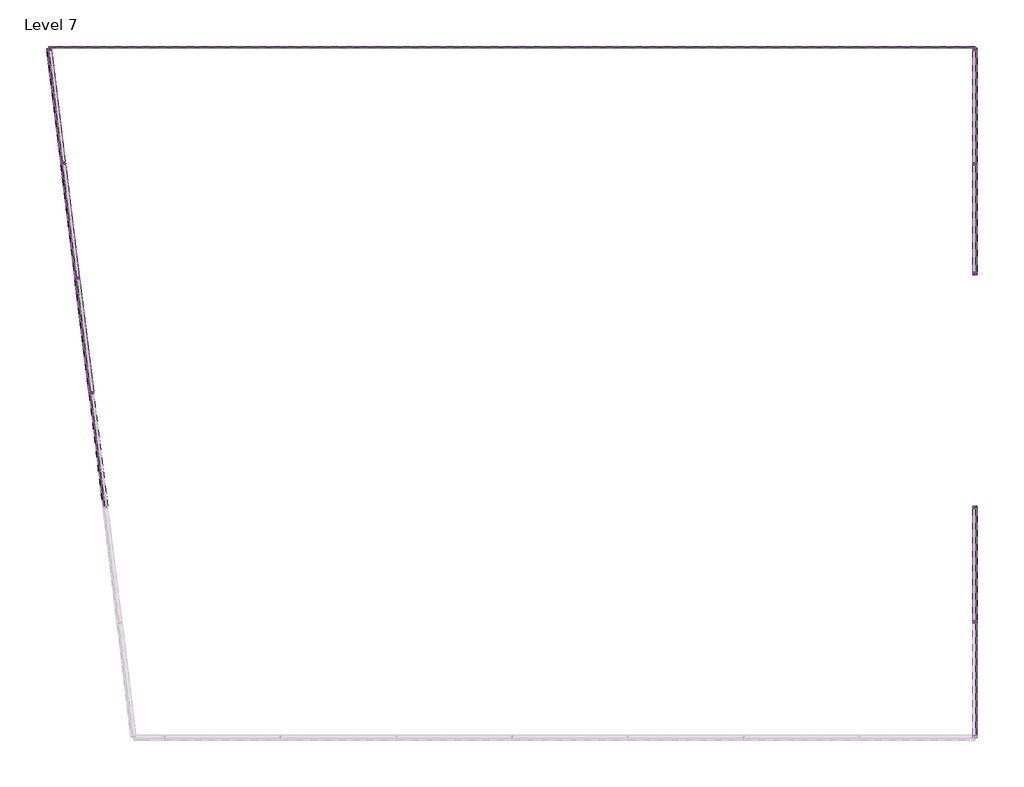
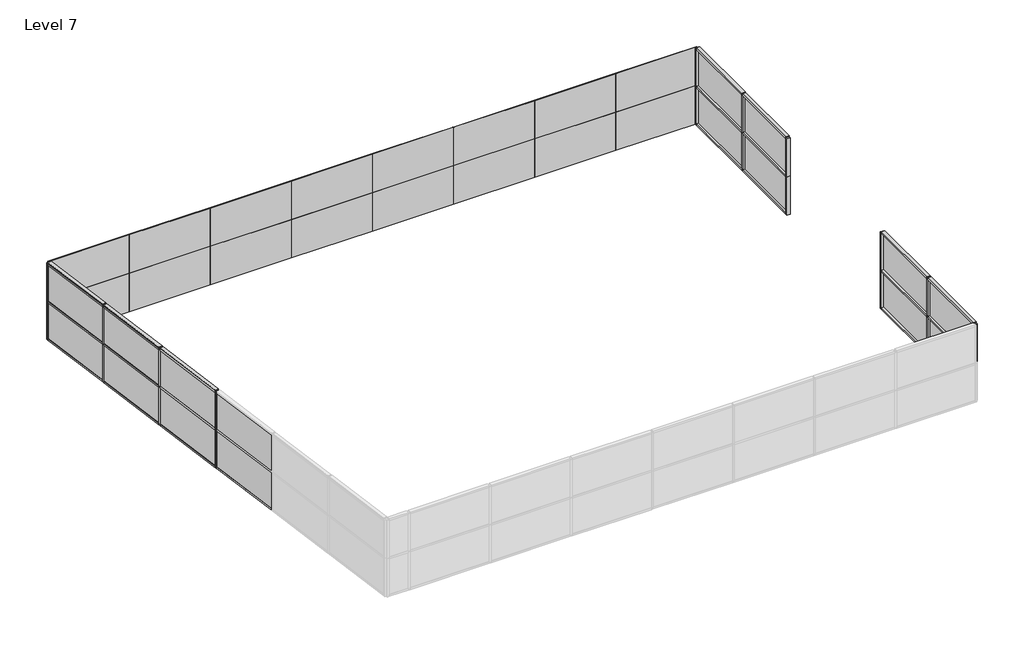
# One storey, part 2 of 2: 54 members, 40 plates.
"""IFC4 building model written with IfcOpenShell, lengths in millimetres."""

from ifc_helpers import new_model, si_unit, origin, place, context, project, spatial, transform, mapped, element, save
from components import member_71c27fd2, member_daa7a266, member_82905deb, member_19d0a4ec, member_8cef0660, member_db480205, member_4491d118, member_1b94d493, member_46bdb8c2, system_panel_glazed_1e57f9bb, system_panel_glazed_37f15d2e, system_panel_glazed_3620f98e, system_panel_glazed_e46d4b42, system_panel_glazed_2a6c68b7, system_panel_glazed_7fb1fc2b, system_panel_glazed_d483336f

model = new_model("IFC4")

# Units and contexts
model_context = context("Model", 3, world=origin())
ifc_project = project(units=[si_unit("LENGTHUNIT", "METRE", prefix="MILLI")], contexts=[model_context])

# Site, building, storey
site = spatial("IfcSite", under=ifc_project)
building = spatial("IfcBuilding", under=site)
storey = spatial("IfcBuildingStorey", under=building, Name="Level 7", Elevation=18288.0)

# Members
placement = place(None, origin())
member_shape = member_71c27fd2(model_context)
element("IfcMember", 1, ObjectType="Rectangular Mullion : 2.5\" x 5\" rectangular", at=placement, inside=storey, context=model_context, shape_type="MappedRepresentation", body=[
    mapped(member_shape, transform((-10473.7456604, 11109.5209701, 18288.0), x_axis=(0.0, 0.0, -1.0), y_axis=(-0.9925461516413222, -0.12186934340514599, 0.0), z_axis=(-0.12186934340514599, 0.9925461516413222, 0.0))),
])
element("IfcMember", 2, ObjectType="Rectangular Mullion : 2.5\" x 5\" rectangular", at=placement, inside=storey, context=model_context, shape_type="MappedRepresentation", body=[
    mapped(member_shape, transform((13902.5156363, -3899.3863708, 18288.0), x_axis=(0.0, 0.0, -1.0), y_axis=(1.0, 0.0, 0.0), z_axis=(0.0, -1.0, 0.0))),
])
element("IfcMember", 3, ObjectType="Rectangular Mullion : 2.5\" x 5\" rectangular", at=placement, inside=storey, context=model_context, shape_type="MappedRepresentation", body=[
    mapped(member_shape, transform((13902.5156363, 8156.2976505, 18288.0), x_axis=(0.0, 0.0, -1.0), y_axis=(1.0, 0.0, 0.0), z_axis=(0.0, -1.0, 0.0))),
])
member_2_shape = member_daa7a266(model_context)
element("IfcMember", 4, ObjectType="Rectangular Mullion : 2.5\" x 5\" rectangular", at=placement, inside=storey, context=model_context, shape_type="MappedRepresentation", body=[
    mapped(member_2_shape, transform((-10113.8959567, 8178.7803212, 21336.0), x_axis=(0.0, 0.0, 1.0), y_axis=(-0.9925461516413222, -0.12186934340514625, 0.0), z_axis=(0.12186934340514625, -0.9925461516413222, 0.0))),
])
member_3_shape = member_82905deb(model_context)
element("IfcMember", 5, ObjectType="Rectangular Mullion : 2.5\" x 5\" rectangular", at=placement, inside=storey, context=model_context, shape_type="MappedRepresentation", body=[
    mapped(member_3_shape, transform((-9367.1110876, 2096.7056405, 21336.0), x_axis=(-0.1218693434051459, 0.9925461516413222, 0.0), y_axis=(-0.9925461516413222, -0.1218693434051459, 0.0), z_axis=(0.0, 0.0, 1.0))),
])
element("IfcMember", 6, ObjectType="Rectangular Mullion : 2.5\" x 5\" rectangular", at=placement, inside=storey, context=model_context, shape_type="MappedRepresentation", body=[
    mapped(member_3_shape, transform((-9738.5688463, 5121.9863107, 21336.0), x_axis=(-0.1218693434051459, 0.9925461516413222, 0.0), y_axis=(-0.9925461516413222, -0.1218693434051459, 0.0), z_axis=(0.0, 0.0, 1.0))),
])
element("IfcMember", 7, ObjectType="Rectangular Mullion : 2.5\" x 5\" rectangular", at=placement, inside=storey, context=model_context, shape_type="MappedRepresentation", body=[
    mapped(member_3_shape, transform((-10110.026605, 8147.2669809, 21336.0), x_axis=(-0.1218693434051459, 0.9925461516413222, 0.0), y_axis=(-0.9925461516413222, -0.1218693434051459, 0.0), z_axis=(0.0, 0.0, 1.0))),
])
member_4_shape = member_19d0a4ec(model_context)
element("IfcMember", 8, ObjectType="Rectangular Mullion : 2.5\" x 5\" rectangular", at=placement, inside=storey, context=model_context, shape_type="MappedRepresentation", body=[
    mapped(member_4_shape, transform((-10113.8959567, 8178.7803212, 19812.0), x_axis=(0.0, 0.0, 1.0), y_axis=(-0.9925461516413223, -0.12186934340514552, 0.0), z_axis=(0.1218693434051455, -0.9925461516413222, 0.0))),
])
element("IfcMember", 9, ObjectType="Rectangular Mullion : 2.5\" x 5\" rectangular", at=placement, inside=storey, context=model_context, shape_type="MappedRepresentation", body=[
    mapped(member_4_shape, transform((-10113.8959567, 8178.7803212, 19812.0), x_axis=(0.0, 0.0, 1.0), y_axis=(-0.9925461516413222, -0.12186934340514599, 0.0), z_axis=(0.12186934340514599, -0.9925461516413222, 0.0))),
])
element("IfcMember", 10, ObjectType="Rectangular Mullion : 2.5\" x 5\" rectangular", at=placement, inside=storey, context=model_context, shape_type="MappedRepresentation", body=[
    mapped(member_4_shape, transform((-10113.8959567, 8178.7803212, 21336.0), x_axis=(0.0, 0.0, 1.0), y_axis=(-0.9925461516413222, -0.12186934340514599, 0.0), z_axis=(0.12186934340514599, -0.9925461516413222, 0.0))),
])
element("IfcMember", 11, ObjectType="Rectangular Mullion : 2.5\" x 5\" rectangular", at=placement, inside=storey, context=model_context, shape_type="MappedRepresentation", body=[
    mapped(member_4_shape, transform((13902.5156363, -946.6363705, 19812.0), x_axis=(0.0, 0.0, 1.0), y_axis=(1.0, 0.0, 0.0), z_axis=(0.0, 1.0, 0.0))),
])
element("IfcMember", 12, ObjectType="Rectangular Mullion : 2.5\" x 5\" rectangular", at=placement, inside=storey, context=model_context, shape_type="MappedRepresentation", body=[
    mapped(member_4_shape, transform((13902.5156363, -3962.8863708, 19812.0), x_axis=(0.0, 0.0, 1.0), y_axis=(1.0, 0.0, 0.0), z_axis=(0.0, 1.0, 0.0))),
])
element("IfcMember", 13, ObjectType="Rectangular Mullion : 2.5\" x 5\" rectangular", at=placement, inside=storey, context=model_context, shape_type="MappedRepresentation", body=[
    mapped(member_4_shape, transform((13902.5156363, -946.6363705, 21336.0), x_axis=(0.0, 0.0, 1.0), y_axis=(1.0, 0.0, 0.0), z_axis=(0.0, 1.0, 0.0))),
])
element("IfcMember", 14, ObjectType="Rectangular Mullion : 2.5\" x 5\" rectangular", at=placement, inside=storey, context=model_context, shape_type="MappedRepresentation", body=[
    mapped(member_4_shape, transform((13902.5156363, -3962.8863708, 21336.0), x_axis=(0.0, 0.0, 1.0), y_axis=(1.0, 0.0, 0.0), z_axis=(0.0, 1.0, 0.0))),
])
element("IfcMember", 15, ObjectType="Rectangular Mullion : 2.5\" x 5\" rectangular", at=placement, inside=storey, context=model_context, shape_type="MappedRepresentation", body=[
    mapped(member_4_shape, transform((13902.5156363, 11109.0476508, 19812.0), x_axis=(0.0, 0.0, 1.0), y_axis=(1.0, 0.0, 0.0), z_axis=(0.0, 1.0, 0.0))),
])
element("IfcMember", 16, ObjectType="Rectangular Mullion : 2.5\" x 5\" rectangular", at=placement, inside=storey, context=model_context, shape_type="MappedRepresentation", body=[
    mapped(member_4_shape, transform((13902.5156363, 11109.0476508, 21336.0), x_axis=(0.0, 0.0, 1.0), y_axis=(1.0, 0.0, 0.0), z_axis=(0.0, 1.0, 0.0))),
])
member_5_shape = member_8cef0660(model_context)
element("IfcMember", 17, ObjectType="Rectangular Mullion : 2.5\" x 5\" rectangular", at=placement, inside=storey, context=model_context, shape_type="MappedRepresentation", body=[
    mapped(member_5_shape, transform((-9370.9804393, 2128.2189808, 19812.0), x_axis=(0.0, 0.0, 1.0), y_axis=(-0.9925461516413222, -0.12186934340514592, 0.0), z_axis=(0.12186934340514592, -0.9925461516413222, 0.0))),
])
element("IfcMember", 18, ObjectType="Rectangular Mullion : 2.5\" x 5\" rectangular", at=placement, inside=storey, context=model_context, shape_type="MappedRepresentation", body=[
    mapped(member_5_shape, transform((-9742.438198, 5153.499651, 19812.0), x_axis=(0.0, 0.0, 1.0), y_axis=(-0.9925461516413222, -0.12186934340514602, 0.0), z_axis=(0.12186934340514602, -0.9925461516413222, 0.0))),
])
element("IfcMember", 19, ObjectType="Rectangular Mullion : 2.5\" x 5\" rectangular", at=placement, inside=storey, context=model_context, shape_type="MappedRepresentation", body=[
    mapped(member_5_shape, transform((-9370.9804393, 2128.2189808, 19812.0), x_axis=(0.0, 0.0, 1.0), y_axis=(-0.9925461516413222, -0.12186934340514592, 0.0), z_axis=(0.12186934340514592, -0.9925461516413222, 0.0))),
])
element("IfcMember", 20, ObjectType="Rectangular Mullion : 2.5\" x 5\" rectangular", at=placement, inside=storey, context=model_context, shape_type="MappedRepresentation", body=[
    mapped(member_5_shape, transform((-9742.438198, 5153.499651, 19812.0), x_axis=(0.0, 0.0, 1.0), y_axis=(-0.9925461516413222, -0.1218693434051457, 0.0), z_axis=(0.1218693434051457, -0.9925461516413222, 0.0))),
])
element("IfcMember", 21, ObjectType="Rectangular Mullion : 2.5\" x 5\" rectangular", at=placement, inside=storey, context=model_context, shape_type="MappedRepresentation", body=[
    mapped(member_5_shape, transform((-9370.9804393, 2128.2189808, 21336.0), x_axis=(0.0, 0.0, 1.0), y_axis=(-0.9925461516413222, -0.12186934340514595, 0.0), z_axis=(0.12186934340514595, -0.9925461516413222, 0.0))),
])
element("IfcMember", 22, ObjectType="Rectangular Mullion : 2.5\" x 5\" rectangular", at=placement, inside=storey, context=model_context, shape_type="MappedRepresentation", body=[
    mapped(member_5_shape, transform((-9742.438198, 5153.499651, 21336.0), x_axis=(0.0, 0.0, 1.0), y_axis=(-0.9925461516413222, -0.12186934340514606, 0.0), z_axis=(0.12186934340514606, -0.9925461516413222, 0.0))),
])
member_6_shape = member_db480205(model_context)
element("IfcMember", 23, ObjectType="Rectangular Mullion : 2.5\" x 5\" rectangular", at=placement, inside=storey, context=model_context, shape_type="MappedRepresentation", body=[
    mapped(member_6_shape, transform((-9363.241736, 2065.1923001, 18288.0), x_axis=(0.0, 0.0, -1.0), y_axis=(-0.9925461516413223, -0.12186934340514559, 0.0), z_axis=(-0.12186934340514559, 0.9925461516413223, 0.0))),
])
element("IfcMember", 24, ObjectType="Rectangular Mullion : 2.5\" x 5\" rectangular", at=placement, inside=storey, context=model_context, shape_type="MappedRepresentation", body=[
    mapped(member_6_shape, transform((-9734.6994947, 5090.4729703, 18288.0), x_axis=(0.0, 0.0, -1.0), y_axis=(-0.9925461516413222, -0.12186934340514592, 0.0), z_axis=(-0.12186934340514592, 0.9925461516413222, 0.0))),
])
element("IfcMember", 25, ObjectType="Rectangular Mullion : 2.5\" x 5\" rectangular", at=placement, inside=storey, context=model_context, shape_type="MappedRepresentation", body=[
    mapped(member_6_shape, transform((-10106.1572534, 8115.7536405, 18288.0), x_axis=(0.0, 0.0, -1.0), y_axis=(-0.9925461516413222, -0.12186934340514606, 0.0), z_axis=(-0.12186934340514606, 0.9925461516413222, 0.0))),
])
element("IfcMember", 26, ObjectType="Rectangular Mullion : 2.5\" x 5\" rectangular", at=placement, inside=storey, context=model_context, shape_type="MappedRepresentation", body=[
    mapped(member_6_shape, transform((-9370.9804393, 2128.2189808, 21336.0), x_axis=(0.0, 0.0, 1.0), y_axis=(-0.9925461516413222, -0.12186934340514592, 0.0), z_axis=(0.12186934340514592, -0.9925461516413222, 0.0))),
])
element("IfcMember", 27, ObjectType="Rectangular Mullion : 2.5\" x 5\" rectangular", at=placement, inside=storey, context=model_context, shape_type="MappedRepresentation", body=[
    mapped(member_6_shape, transform((-9742.438198, 5153.499651, 21336.0), x_axis=(0.0, 0.0, 1.0), y_axis=(-0.9925461516413222, -0.1218693434051457, 0.0), z_axis=(0.1218693434051457, -0.9925461516413222, 0.0))),
])
element("IfcMember", 28, ObjectType="Rectangular Mullion : 2.5\" x 5\" rectangular", at=placement, inside=storey, context=model_context, shape_type="MappedRepresentation", body=[
    mapped(member_3_shape, transform((-9367.1110876, 2096.7056405, 19812.0), x_axis=(-0.1218693434051459, 0.9925461516413222, 0.0), y_axis=(-0.9925461516413222, -0.1218693434051459, 0.0), z_axis=(0.0, 0.0, 1.0))),
])
element("IfcMember", 29, ObjectType="Rectangular Mullion : 2.5\" x 5\" rectangular", at=placement, inside=storey, context=model_context, shape_type="MappedRepresentation", body=[
    mapped(member_3_shape, transform((-9738.5688463, 5121.9863107, 19812.0), x_axis=(-0.1218693434051459, 0.9925461516413222, 0.0), y_axis=(-0.9925461516413222, -0.1218693434051459, 0.0), z_axis=(0.0, 0.0, 1.0))),
])
element("IfcMember", 30, ObjectType="Rectangular Mullion : 2.5\" x 5\" rectangular", at=placement, inside=storey, context=model_context, shape_type="MappedRepresentation", body=[
    mapped(member_3_shape, transform((-10110.026605, 8147.2669809, 19812.0), x_axis=(-0.1218693434051459, 0.9925461516413222, 0.0), y_axis=(-0.9925461516413222, -0.1218693434051459, 0.0), z_axis=(0.0, 0.0, 1.0))),
])
element("IfcMember", 31, ObjectType="Rectangular Mullion : 2.5\" x 5\" rectangular", at=placement, inside=storey, context=model_context, shape_type="MappedRepresentation", body=[
    mapped(member_3_shape, transform((13902.5156363, -3931.1363708, 19812.0), x_axis=(0.0, -1.0, 0.0), y_axis=(1.0, 0.0, 0.0), z_axis=(0.0, 0.0, 1.0))),
])
element("IfcMember", 32, ObjectType="Rectangular Mullion : 2.5\" x 5\" rectangular", at=placement, inside=storey, context=model_context, shape_type="MappedRepresentation", body=[
    mapped(member_3_shape, transform((13902.5156363, 8124.5476505, 19812.0), x_axis=(0.0, -1.0, 0.0), y_axis=(1.0, 0.0, 0.0), z_axis=(0.0, 0.0, 1.0))),
])
element("IfcMember", 33, ObjectType="Rectangular Mullion : 2.5\" x 5\" rectangular", at=placement, inside=storey, context=model_context, shape_type="MappedRepresentation", body=[
    mapped(member_3_shape, transform((-9367.1110876, 2096.7056405, 19812.0), x_axis=(-0.1218693434051459, 0.9925461516413222, 0.0), y_axis=(-0.9925461516413222, -0.1218693434051459, 0.0), z_axis=(0.0, 0.0, 1.0))),
])
element("IfcMember", 34, ObjectType="Rectangular Mullion : 2.5\" x 5\" rectangular", at=placement, inside=storey, context=model_context, shape_type="MappedRepresentation", body=[
    mapped(member_3_shape, transform((-9738.5688463, 5121.9863107, 19812.0), x_axis=(-0.1218693434051459, 0.9925461516413222, 0.0), y_axis=(-0.9925461516413222, -0.1218693434051459, 0.0), z_axis=(0.0, 0.0, 1.0))),
])
element("IfcMember", 35, ObjectType="Rectangular Mullion : 2.5\" x 5\" rectangular", at=placement, inside=storey, context=model_context, shape_type="MappedRepresentation", body=[
    mapped(member_3_shape, transform((-10110.026605, 8147.2669809, 19812.0), x_axis=(-0.1218693434051459, 0.9925461516413222, 0.0), y_axis=(-0.9925461516413222, -0.1218693434051459, 0.0), z_axis=(0.0, 0.0, 1.0))),
])
element("IfcMember", 36, ObjectType="Rectangular Mullion : 2.5\" x 5\" rectangular", at=placement, inside=storey, context=model_context, shape_type="MappedRepresentation", body=[
    mapped(member_3_shape, transform((-9367.1110876, 2096.7056405, 21336.0), x_axis=(-0.1218693434051459, 0.9925461516413222, 0.0), y_axis=(-0.9925461516413222, -0.1218693434051459, 0.0), z_axis=(0.0, 0.0, 1.0))),
])
element("IfcMember", 37, ObjectType="Rectangular Mullion : 2.5\" x 5\" rectangular", at=placement, inside=storey, context=model_context, shape_type="MappedRepresentation", body=[
    mapped(member_3_shape, transform((-9738.5688463, 5121.9863107, 21336.0), x_axis=(-0.1218693434051459, 0.9925461516413222, 0.0), y_axis=(-0.9925461516413222, -0.1218693434051459, 0.0), z_axis=(0.0, 0.0, 1.0))),
])
element("IfcMember", 38, ObjectType="Rectangular Mullion : 2.5\" x 5\" rectangular", at=placement, inside=storey, context=model_context, shape_type="MappedRepresentation", body=[
    mapped(member_3_shape, transform((-10110.026605, 8147.2669809, 21336.0), x_axis=(-0.1218693434051459, 0.9925461516413222, 0.0), y_axis=(-0.9925461516413222, -0.1218693434051459, 0.0), z_axis=(0.0, 0.0, 1.0))),
])
element("IfcMember", 39, ObjectType="Rectangular Mullion : 2.5\" x 5\" rectangular", at=placement, inside=storey, context=model_context, shape_type="MappedRepresentation", body=[
    mapped(member_3_shape, transform((13902.5156363, -3931.1363708, 21336.0), x_axis=(0.0, -1.0, 0.0), y_axis=(1.0, 0.0, 0.0), z_axis=(0.0, 0.0, 1.0))),
])
element("IfcMember", 40, ObjectType="Rectangular Mullion : 2.5\" x 5\" rectangular", at=placement, inside=storey, context=model_context, shape_type="MappedRepresentation", body=[
    mapped(member_3_shape, transform((13902.5156363, 8124.5476505, 21336.0), x_axis=(0.0, -1.0, 0.0), y_axis=(1.0, 0.0, 0.0), z_axis=(0.0, 0.0, 1.0))),
])
member_7_shape = member_4491d118(model_context)
element("IfcMember", 41, ObjectType="Rectangular Mullion : 2.5\" x 5\" rectangular", at=placement, inside=storey, context=model_context, shape_type="MappedRepresentation", body=[
    mapped(member_7_shape, transform((-10481.4843637, 11172.5476508, 21336.0), x_axis=(-0.1218693434051459, 0.9925461516413222, 0.0), y_axis=(-0.9925461516413222, -0.1218693434051459, 0.0), z_axis=(0.0, 0.0, 1.0))),
])
element("IfcMember", 42, ObjectType="Rectangular Mullion : 2.5\" x 5\" rectangular", at=placement, inside=storey, context=model_context, shape_type="MappedRepresentation", body=[
    mapped(member_7_shape, transform((13902.5156363, -883.1363705, 18288.0), x_axis=(0.0, 1.0, 0.0), y_axis=(1.0, 0.0, 0.0), z_axis=(0.0, 0.0, -1.0))),
])
element("IfcMember", 43, ObjectType="Rectangular Mullion : 2.5\" x 5\" rectangular", at=placement, inside=storey, context=model_context, shape_type="MappedRepresentation", body=[
    mapped(member_7_shape, transform((13902.5156363, 11172.5476508, 18288.0), x_axis=(0.0, 1.0, 0.0), y_axis=(1.0, 0.0, 0.0), z_axis=(0.0, 0.0, -1.0))),
])
element("IfcMember", 44, ObjectType="Rectangular Mullion : 2.5\" x 5\" rectangular", at=placement, inside=storey, context=model_context, shape_type="MappedRepresentation", body=[
    mapped(member_7_shape, transform((13902.5156363, -883.1363705, 19812.0), x_axis=(0.0, 1.0, 0.0), y_axis=(1.0, 0.0, 0.0), z_axis=(0.0, 0.0, -1.0))),
])
element("IfcMember", 45, ObjectType="Rectangular Mullion : 2.5\" x 5\" rectangular", at=placement, inside=storey, context=model_context, shape_type="MappedRepresentation", body=[
    mapped(member_7_shape, transform((13902.5156363, 11172.5476508, 19812.0), x_axis=(0.0, 1.0, 0.0), y_axis=(1.0, 0.0, 0.0), z_axis=(0.0, 0.0, -1.0))),
])
element("IfcMember", 46, ObjectType="Rectangular Mullion : 2.5\" x 5\" rectangular", at=placement, inside=storey, context=model_context, shape_type="MappedRepresentation", body=[
    mapped(member_7_shape, transform((-10481.4843637, 11172.5476508, 19812.0), x_axis=(-0.1218693434051459, 0.9925461516413222, 0.0), y_axis=(-0.9925461516413222, -0.1218693434051459, 0.0), z_axis=(0.0, 0.0, 1.0))),
])
element("IfcMember", 47, ObjectType="Rectangular Mullion : 2.5\" x 5\" rectangular", at=placement, inside=storey, context=model_context, shape_type="MappedRepresentation", body=[
    mapped(member_7_shape, transform((13902.5156363, 5212.8636295, 19812.0), x_axis=(0.0, -1.0, 0.0), y_axis=(1.0, 0.0, 0.0), z_axis=(0.0, 0.0, 1.0))),
])
element("IfcMember", 48, ObjectType="Rectangular Mullion : 2.5\" x 5\" rectangular", at=placement, inside=storey, context=model_context, shape_type="MappedRepresentation", body=[
    mapped(member_7_shape, transform((-10481.4843637, 11172.5476508, 19812.0), x_axis=(-0.1218693434051459, 0.9925461516413222, 0.0), y_axis=(-0.9925461516413222, -0.1218693434051459, 0.0), z_axis=(0.0, 0.0, 1.0))),
])
element("IfcMember", 49, ObjectType="Rectangular Mullion : 2.5\" x 5\" rectangular", at=placement, inside=storey, context=model_context, shape_type="MappedRepresentation", body=[
    mapped(member_7_shape, transform((-10481.4843637, 11172.5476508, 21336.0), x_axis=(-0.1218693434051459, 0.9925461516413222, 0.0), y_axis=(-0.9925461516413222, -0.1218693434051459, 0.0), z_axis=(0.0, 0.0, 1.0))),
])
element("IfcMember", 50, ObjectType="Rectangular Mullion : 2.5\" x 5\" rectangular", at=placement, inside=storey, context=model_context, shape_type="MappedRepresentation", body=[
    mapped(member_7_shape, transform((13902.5156363, -6979.1363705, 21336.0), x_axis=(0.0, -1.0, 0.0), y_axis=(1.0, 0.0, 0.0), z_axis=(0.0, 0.0, 1.0))),
])
element("IfcMember", 51, ObjectType="Rectangular Mullion : 2.5\" x 5\" rectangular", at=placement, inside=storey, context=model_context, shape_type="MappedRepresentation", body=[
    mapped(member_7_shape, transform((13902.5156363, 5212.8636295, 21336.0), x_axis=(0.0, -1.0, 0.0), y_axis=(1.0, 0.0, 0.0), z_axis=(0.0, 0.0, 1.0))),
])
member_8_shape = member_1b94d493(model_context)
element("IfcMember", 52, ObjectType="Rectangular Mullion : 2.5\" x 5\" rectangular", at=placement, inside=storey, context=model_context, shape_type="MappedRepresentation", body=[
    mapped(member_8_shape, transform((13902.5156363, 5276.3636295, 18288.0), x_axis=(0.0, 0.0, -1.0), y_axis=(1.0, 0.0, 0.0), z_axis=(0.0, -1.0, 0.0))),
])
member_9_shape = member_46bdb8c2(model_context)
element("IfcMember", 53, ObjectType="Rectangular Mullion : 2.5\" x 5\" rectangular", at=placement, inside=storey, context=model_context, shape_type="MappedRepresentation", body=[
    mapped(member_9_shape, transform((13902.5156363, 8092.7976505, 19812.0), x_axis=(0.0, 0.0, 1.0), y_axis=(1.0, 0.0, 0.0), z_axis=(0.0, 1.0, 0.0))),
])
element("IfcMember", 54, ObjectType="Rectangular Mullion : 2.5\" x 5\" rectangular", at=placement, inside=storey, context=model_context, shape_type="MappedRepresentation", body=[
    mapped(member_9_shape, transform((13902.5156363, 8092.7976505, 21336.0), x_axis=(0.0, 0.0, 1.0), y_axis=(1.0, 0.0, 0.0), z_axis=(0.0, 1.0, 0.0))),
])

# Plates
system_panel_glazed_shape = system_panel_glazed_1e57f9bb(model_context)
element("IfcPlate", 55, ObjectType="System Panel : Glazed", at=placement, inside=storey, context=model_context, shape_type="MappedRepresentation", body=[
    mapped(system_panel_glazed_shape, transform((-8957.4843636, 11172.5476508, 18288.0), x_axis=(1.0, 0.0, 0.0), y_axis=(0.0, 1.0, 0.0), z_axis=(0.0, 0.0, 1.0))),
])
element("IfcPlate", 56, ObjectType="System Panel : Glazed", at=placement, inside=storey, context=model_context, shape_type="MappedRepresentation", body=[
    mapped(system_panel_glazed_shape, transform((-5909.4843634, 11172.5476508, 18288.0), x_axis=(1.0, 0.0, 0.0), y_axis=(0.0, 1.0, 0.0), z_axis=(0.0, 0.0, 1.0))),
])
element("IfcPlate", 57, ObjectType="System Panel : Glazed", at=placement, inside=storey, context=model_context, shape_type="MappedRepresentation", body=[
    mapped(system_panel_glazed_shape, transform((-2861.4843634, 11172.5476508, 18288.0), x_axis=(1.0, 0.0, 0.0), y_axis=(0.0, 1.0, 0.0), z_axis=(0.0, 0.0, 1.0))),
])
element("IfcPlate", 58, ObjectType="System Panel : Glazed", at=placement, inside=storey, context=model_context, shape_type="MappedRepresentation", body=[
    mapped(system_panel_glazed_shape, transform((186.5156366, 11172.5476508, 18288.0), x_axis=(1.0, 0.0, 0.0), y_axis=(0.0, 1.0, 0.0), z_axis=(0.0, 0.0, 1.0))),
])
element("IfcPlate", 59, ObjectType="System Panel : Glazed", at=placement, inside=storey, context=model_context, shape_type="MappedRepresentation", body=[
    mapped(system_panel_glazed_shape, transform((3234.5156366, 11172.5476508, 18288.0), x_axis=(1.0, 0.0, 0.0), y_axis=(0.0, 1.0, 0.0), z_axis=(0.0, 0.0, 1.0))),
])
element("IfcPlate", 60, ObjectType="System Panel : Glazed", at=placement, inside=storey, context=model_context, shape_type="MappedRepresentation", body=[
    mapped(system_panel_glazed_shape, transform((6282.5156366, 11172.5476508, 18288.0), x_axis=(1.0, 0.0, 0.0), y_axis=(0.0, 1.0, 0.0), z_axis=(0.0, 0.0, 1.0))),
])
element("IfcPlate", 61, ObjectType="System Panel : Glazed", at=placement, inside=storey, context=model_context, shape_type="MappedRepresentation", body=[
    mapped(system_panel_glazed_shape, transform((9330.5156366, 11172.5476508, 18288.0), x_axis=(1.0, 0.0, 0.0), y_axis=(0.0, 1.0, 0.0), z_axis=(0.0, 0.0, 1.0))),
])
element("IfcPlate", 62, ObjectType="System Panel : Glazed", at=placement, inside=storey, context=model_context, shape_type="MappedRepresentation", body=[
    mapped(system_panel_glazed_shape, transform((12378.5156364, 11172.5476508, 18288.0), x_axis=(1.0, 0.0, 0.0), y_axis=(0.0, 1.0, 0.0), z_axis=(0.0, 0.0, 1.0))),
])
element("IfcPlate", 63, ObjectType="System Panel : Glazed", at=placement, inside=storey, context=model_context, shape_type="MappedRepresentation", body=[
    mapped(system_panel_glazed_shape, transform((-8957.4843636, 11172.5476508, 19812.0), x_axis=(1.0, 0.0, 0.0), y_axis=(0.0, 1.0, 0.0), z_axis=(0.0, 0.0, 1.0))),
])
element("IfcPlate", 64, ObjectType="System Panel : Glazed", at=placement, inside=storey, context=model_context, shape_type="MappedRepresentation", body=[
    mapped(system_panel_glazed_shape, transform((-5909.4843634, 11172.5476508, 19812.0), x_axis=(1.0, 0.0, 0.0), y_axis=(0.0, 1.0, 0.0), z_axis=(0.0, 0.0, 1.0))),
])
element("IfcPlate", 65, ObjectType="System Panel : Glazed", at=placement, inside=storey, context=model_context, shape_type="MappedRepresentation", body=[
    mapped(system_panel_glazed_shape, transform((-2861.4843634, 11172.5476508, 19812.0), x_axis=(1.0, 0.0, 0.0), y_axis=(0.0, 1.0, 0.0), z_axis=(0.0, 0.0, 1.0))),
])
element("IfcPlate", 66, ObjectType="System Panel : Glazed", at=placement, inside=storey, context=model_context, shape_type="MappedRepresentation", body=[
    mapped(system_panel_glazed_shape, transform((186.5156366, 11172.5476508, 19812.0), x_axis=(1.0, 0.0, 0.0), y_axis=(0.0, 1.0, 0.0), z_axis=(0.0, 0.0, 1.0))),
])
element("IfcPlate", 67, ObjectType="System Panel : Glazed", at=placement, inside=storey, context=model_context, shape_type="MappedRepresentation", body=[
    mapped(system_panel_glazed_shape, transform((3234.5156366, 11172.5476508, 19812.0), x_axis=(1.0, 0.0, 0.0), y_axis=(0.0, 1.0, 0.0), z_axis=(0.0, 0.0, 1.0))),
])
element("IfcPlate", 68, ObjectType="System Panel : Glazed", at=placement, inside=storey, context=model_context, shape_type="MappedRepresentation", body=[
    mapped(system_panel_glazed_shape, transform((6282.5156366, 11172.5476508, 19812.0), x_axis=(1.0, 0.0, 0.0), y_axis=(0.0, 1.0, 0.0), z_axis=(0.0, 0.0, 1.0))),
])
element("IfcPlate", 69, ObjectType="System Panel : Glazed", at=placement, inside=storey, context=model_context, shape_type="MappedRepresentation", body=[
    mapped(system_panel_glazed_shape, transform((9330.5156366, 11172.5476508, 19812.0), x_axis=(1.0, 0.0, 0.0), y_axis=(0.0, 1.0, 0.0), z_axis=(0.0, 0.0, 1.0))),
])
element("IfcPlate", 70, ObjectType="System Panel : Glazed", at=placement, inside=storey, context=model_context, shape_type="MappedRepresentation", body=[
    mapped(system_panel_glazed_shape, transform((12378.5156364, 11172.5476508, 19812.0), x_axis=(1.0, 0.0, 0.0), y_axis=(0.0, 1.0, 0.0), z_axis=(0.0, 0.0, 1.0))),
])
system_panel_glazed_2_shape = system_panel_glazed_37f15d2e(model_context)
element("IfcPlate", 71, ObjectType="System Panel : Glazed", at=placement, inside=storey, context=model_context, shape_type="MappedRepresentation", body=[
    mapped(system_panel_glazed_2_shape, transform((13902.5156363, -2423.0113706, 18351.5), x_axis=(0.0, -1.0, 0.0), y_axis=(1.0, 0.0, 0.0), z_axis=(0.0, 0.0, 1.0))),
])
element("IfcPlate", 72, ObjectType="System Panel : Glazed", at=placement, inside=storey, context=model_context, shape_type="MappedRepresentation", body=[
    mapped(system_panel_glazed_2_shape, transform((13902.5156363, 9632.6726506, 18351.5), x_axis=(0.0, -1.0, 0.0), y_axis=(1.0, 0.0, 0.0), z_axis=(0.0, 0.0, 1.0))),
])
element("IfcPlate", 73, ObjectType="System Panel : Glazed", at=placement, inside=storey, context=model_context, shape_type="MappedRepresentation", body=[
    mapped(system_panel_glazed_2_shape, transform((-10293.8208085, 9644.1506457, 19843.75), x_axis=(-0.1218693434051459, 0.9925461516413222, 0.0), y_axis=(-0.9925461516413222, -0.1218693434051459, 0.0), z_axis=(0.0, 0.0, 1.0))),
])
element("IfcPlate", 74, ObjectType="System Panel : Glazed", at=placement, inside=storey, context=model_context, shape_type="MappedRepresentation", body=[
    mapped(system_panel_glazed_2_shape, transform((-10293.8208085, 9644.1506457, 18351.5), x_axis=(-0.1218693434051459, 0.9925461516413222, 0.0), y_axis=(-0.9925461516413222, -0.1218693434051459, 0.0), z_axis=(0.0, 0.0, 1.0))),
])
element("IfcPlate", 75, ObjectType="System Panel : Glazed", at=placement, inside=storey, context=model_context, shape_type="MappedRepresentation", body=[
    mapped(system_panel_glazed_2_shape, transform((13902.5156363, -5439.2613706, 18351.5), x_axis=(0.0, -1.0, 0.0), y_axis=(1.0, 0.0, 0.0), z_axis=(0.0, 0.0, 1.0))),
])
system_panel_glazed_3_shape = system_panel_glazed_3620f98e(model_context)
element("IfcPlate", 76, ObjectType="System Panel : Glazed", at=placement, inside=storey, context=model_context, shape_type="MappedRepresentation", body=[
    mapped(system_panel_glazed_3_shape, transform((-9181.3822083, 584.0653054, 19843.75), x_axis=(-0.1218693434051459, 0.9925461516413222, 0.0), y_axis=(-0.9925461516413222, -0.1218693434051459, 0.0), z_axis=(0.0, 0.0, 1.0))),
])
element("IfcPlate", 77, ObjectType="System Panel : Glazed", at=placement, inside=storey, context=model_context, shape_type="MappedRepresentation", body=[
    mapped(system_panel_glazed_3_shape, transform((-9552.839967, 3609.3459756, 19843.75), x_axis=(-0.1218693434051459, 0.9925461516413222, 0.0), y_axis=(-0.9925461516413222, -0.1218693434051459, 0.0), z_axis=(0.0, 0.0, 1.0))),
])
element("IfcPlate", 78, ObjectType="System Panel : Glazed", at=placement, inside=storey, context=model_context, shape_type="MappedRepresentation", body=[
    mapped(system_panel_glazed_3_shape, transform((-9924.2977257, 6634.6266458, 19843.75), x_axis=(-0.1218693434051459, 0.9925461516413222, 0.0), y_axis=(-0.9925461516413222, -0.1218693434051459, 0.0), z_axis=(0.0, 0.0, 1.0))),
])
element("IfcPlate", 79, ObjectType="System Panel : Glazed", at=placement, inside=storey, context=model_context, shape_type="MappedRepresentation", body=[
    mapped(system_panel_glazed_3_shape, transform((-9181.3822083, 584.0653054, 18351.5), x_axis=(-0.1218693434051459, 0.9925461516413222, 0.0), y_axis=(-0.9925461516413222, -0.1218693434051459, 0.0), z_axis=(0.0, 0.0, 1.0))),
])
element("IfcPlate", 80, ObjectType="System Panel : Glazed", at=placement, inside=storey, context=model_context, shape_type="MappedRepresentation", body=[
    mapped(system_panel_glazed_3_shape, transform((-9552.839967, 3609.3459756, 18351.5), x_axis=(-0.1218693434051459, 0.9925461516413222, 0.0), y_axis=(-0.9925461516413222, -0.1218693434051459, 0.0), z_axis=(0.0, 0.0, 1.0))),
])
element("IfcPlate", 81, ObjectType="System Panel : Glazed", at=placement, inside=storey, context=model_context, shape_type="MappedRepresentation", body=[
    mapped(system_panel_glazed_3_shape, transform((-9924.2977257, 6634.6266458, 18351.5), x_axis=(-0.1218693434051459, 0.9925461516413222, 0.0), y_axis=(-0.9925461516413222, -0.1218693434051459, 0.0), z_axis=(0.0, 0.0, 1.0))),
])
system_panel_glazed_4_shape = system_panel_glazed_e46d4b42(model_context)
element("IfcPlate", 82, ObjectType="System Panel : Glazed", at=placement, inside=storey, context=model_context, shape_type="MappedRepresentation", body=[
    mapped(system_panel_glazed_4_shape, transform((-10293.8208085, 9644.1506457, 18319.75), x_axis=(-0.1218693434051459, 0.9925461516413222, 0.0), y_axis=(-0.9925461516413222, -0.1218693434051459, 0.0), z_axis=(0.0, 0.0, 1.0))),
])
element("IfcPlate", 83, ObjectType="System Panel : Glazed", at=placement, inside=storey, context=model_context, shape_type="MappedRepresentation", body=[
    mapped(system_panel_glazed_4_shape, transform((-10293.8208085, 9644.1506457, 19843.75), x_axis=(-0.1218693434051459, 0.9925461516413222, 0.0), y_axis=(-0.9925461516413222, -0.1218693434051459, 0.0), z_axis=(0.0, 0.0, 1.0))),
])
element("IfcPlate", 84, ObjectType="System Panel : Glazed", at=placement, inside=storey, context=model_context, shape_type="MappedRepresentation", body=[
    mapped(system_panel_glazed_4_shape, transform((13902.5156363, -2423.0113706, 19843.75), x_axis=(0.0, -1.0, 0.0), y_axis=(1.0, 0.0, 0.0), z_axis=(0.0, 0.0, 1.0))),
])
element("IfcPlate", 85, ObjectType="System Panel : Glazed", at=placement, inside=storey, context=model_context, shape_type="MappedRepresentation", body=[
    mapped(system_panel_glazed_4_shape, transform((13902.5156363, -5439.2613706, 19843.75), x_axis=(0.0, -1.0, 0.0), y_axis=(1.0, 0.0, 0.0), z_axis=(0.0, 0.0, 1.0))),
])
element("IfcPlate", 86, ObjectType="System Panel : Glazed", at=placement, inside=storey, context=model_context, shape_type="MappedRepresentation", body=[
    mapped(system_panel_glazed_4_shape, transform((13902.5156363, 9632.6726506, 19843.75), x_axis=(0.0, -1.0, 0.0), y_axis=(1.0, 0.0, 0.0), z_axis=(0.0, 0.0, 1.0))),
])
system_panel_glazed_5_shape = system_panel_glazed_2a6c68b7(model_context)
element("IfcPlate", 87, ObjectType="System Panel : Glazed", at=placement, inside=storey, context=model_context, shape_type="MappedRepresentation", body=[
    mapped(system_panel_glazed_5_shape, transform((-9181.3822083, 584.0653054, 18319.75), x_axis=(-0.1218693434051459, 0.9925461516413222, 0.0), y_axis=(-0.9925461516413222, -0.1218693434051459, 0.0), z_axis=(0.0, 0.0, 1.0))),
])
element("IfcPlate", 88, ObjectType="System Panel : Glazed", at=placement, inside=storey, context=model_context, shape_type="MappedRepresentation", body=[
    mapped(system_panel_glazed_5_shape, transform((-9552.839967, 3609.3459756, 18319.75), x_axis=(-0.1218693434051459, 0.9925461516413222, 0.0), y_axis=(-0.9925461516413222, -0.1218693434051459, 0.0), z_axis=(0.0, 0.0, 1.0))),
])
element("IfcPlate", 89, ObjectType="System Panel : Glazed", at=placement, inside=storey, context=model_context, shape_type="MappedRepresentation", body=[
    mapped(system_panel_glazed_5_shape, transform((-9924.2977257, 6634.6266458, 18319.75), x_axis=(-0.1218693434051459, 0.9925461516413222, 0.0), y_axis=(-0.9925461516413222, -0.1218693434051459, 0.0), z_axis=(0.0, 0.0, 1.0))),
])
element("IfcPlate", 90, ObjectType="System Panel : Glazed", at=placement, inside=storey, context=model_context, shape_type="MappedRepresentation", body=[
    mapped(system_panel_glazed_5_shape, transform((-9181.3822083, 584.0653054, 19843.75), x_axis=(-0.1218693434051459, 0.9925461516413222, 0.0), y_axis=(-0.9925461516413222, -0.1218693434051459, 0.0), z_axis=(0.0, 0.0, 1.0))),
])
element("IfcPlate", 91, ObjectType="System Panel : Glazed", at=placement, inside=storey, context=model_context, shape_type="MappedRepresentation", body=[
    mapped(system_panel_glazed_5_shape, transform((-9552.839967, 3609.3459756, 19843.75), x_axis=(-0.1218693434051459, 0.9925461516413222, 0.0), y_axis=(-0.9925461516413222, -0.1218693434051459, 0.0), z_axis=(0.0, 0.0, 1.0))),
])
element("IfcPlate", 92, ObjectType="System Panel : Glazed", at=placement, inside=storey, context=model_context, shape_type="MappedRepresentation", body=[
    mapped(system_panel_glazed_5_shape, transform((-9924.2977257, 6634.6266458, 19843.75), x_axis=(-0.1218693434051459, 0.9925461516413222, 0.0), y_axis=(-0.9925461516413222, -0.1218693434051459, 0.0), z_axis=(0.0, 0.0, 1.0))),
])
system_panel_glazed_6_shape = system_panel_glazed_7fb1fc2b(model_context)
element("IfcPlate", 93, ObjectType="System Panel : Glazed", at=placement, inside=storey, context=model_context, shape_type="MappedRepresentation", body=[
    mapped(system_panel_glazed_6_shape, transform((13902.5156363, 6684.58064, 18351.5), x_axis=(0.0, -1.0, 0.0), y_axis=(1.0, 0.0, 0.0), z_axis=(0.0, 0.0, 1.0))),
])
system_panel_glazed_7_shape = system_panel_glazed_d483336f(model_context)
element("IfcPlate", 94, ObjectType="System Panel : Glazed", at=placement, inside=storey, context=model_context, shape_type="MappedRepresentation", body=[
    mapped(system_panel_glazed_7_shape, transform((13902.5156363, 6684.58064, 19843.75), x_axis=(0.0, -1.0, 0.0), y_axis=(1.0, 0.0, 0.0), z_axis=(0.0, 0.0, 1.0))),
])

save(model, "model.ifc")

# Revit data of these elements
# Type "Rectangular Mullion : 2.5\" x 5\" rectangular"
#   built-in parameter 1007304 = 0.416667 (stored number, unit not read)
#   built-in parameter 1007301 = 0.104167 (stored number, unit not read)
#   built-in parameter 1007300 = 0.104167 (stored number, unit not read)
# Type "System Panel : Glazed"
#   Construction Type Id = "GSP4R"
#   Analytic Construction = "1/8 in Pilkington single glazing"
#   Visual Light Transmittance = 0.9
#   Solar Heat Gain Coefficient = 0.86
#   Heat Transfer Coefficient (U) = 1.18115 BTU/(h·ft²·°F)
#   Define Thermal Properties by = 1
# Elements 1, 2, 3, 4, 5, 6, 7, 8, 9, 10, 11, 12, 13, 14, 15, 16, 17, 18, 19, 20, 21, 22, 23, 24, 25, 26, 27, 28, 29, 30, 31, 32, 33, 34, 35, 36, 37, 38, 39, 40, 41, 42, 43, 44, 45, 46, 47, 48, 49, 50, 51, 52, 53, 54 (IfcMember, "Rectangular Mullion : 2.5\" x 5\" rectangular")
#   Phase Created = New Construction
#   Materials on its faces: "Aluminum"
# Elements 55, 56, 57, 58, 59, 60, 61, 62, 63, 64, 65, 66, 67, 68, 69, 70, 71, 72, 73, 74, 75, 76, 77, 78, 79, 80, 81, 82, 83, 84, 85, 86, 87, 88, 89, 90, 91, 92, 93, 94 (IfcPlate, "System Panel : Glazed")
#   Phase Created = New Construction
#   Materials on its faces: "Glass"
# Materials
#   "Aluminum": class "Metal", colour RGB 247 247 247, transparency 0, Description = "Aluminum 6061", Cost = 0
#   "Glass": class "Glass", colour RGB 0 128 192, transparency 0.75, Description = "Soda Lime Glass", Cost = 0
